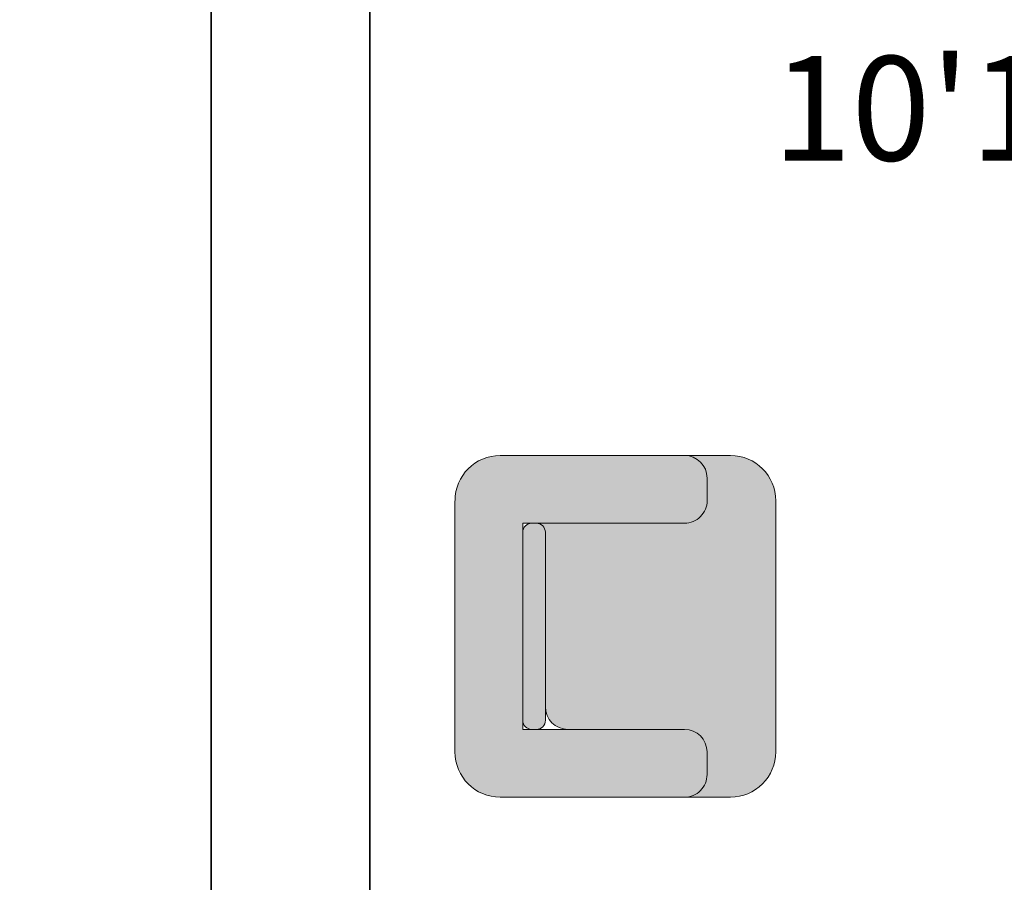
# Model space of a CAD drawing. Units: millimetres. Extents: x 27017497 to 27018854, y 7058029 to 7059154.
# Tile 33 of 91: x 27017621 to 27017677, y 7058337 to 7058386. Entities that reach past the tile are written whole.
import ezdxf

# ---------------------------------------------------------------- set-up
doc = ezdxf.new("R2010")
doc.units = ezdxf.units.MM
for name, color, linetype, lineweight in [('A-ANNO-DIMS', 2, 'Continuous', 18), ('A-FURN', 8, 'Continuous', 18), ('A-WALL', 7, 'Continuous', 35)]:
    doc.layers.add(name, color=color, linetype=linetype, lineweight=lineweight)
doc.layers.add('A-FURN-PATT', color=177, linetype='Continuous', lineweight=13, true_color=0x293189)
doc.styles.get("Standard").update_dxf_attribs({"font": 'arial.ttf'})
doc.dimstyles.get("Standard").update_dxf_attribs({"dimtxt": 0.18, "dimasz": 0.18, "dimexe": 0.18, "dimexo": 0.0625, "dimgap": 0.09, "dimtad": 0, "dimtih": 1, "dimtoh": 1, "dimdec": 4, "dimzin": 0, "dimdsep": 46, "dimtxsty": 'Standard', "dimcen": 0.09, "dimadec": 0, "dimazin": 0, "dimtfac": 1, "dimtdec": 4, "dimtofl": 0, "dimtmove": 0, "dimatfit": 3, "dimfxl": 1, "dimtolj": 1, "dimtzin": 0, "dimarcsym": 0})

# ---------------------------------------------------------------- blocks, each defined once
blk = doc.blocks.new('CHAIR-OCCASIONAL')
for p, q in [((19.599, 18.742), (7.02, 22.21)), ((3.873, 20.423), (0.092, 6.706)), ((4.132, 6.919), (7.234, 18.169)), ((5.25, 10.974), (7.234, 18.169)), ((16.064, 15.735), (7.234, 18.169)), ((7.234, 18.169), (16.064, 15.735)), ((7.234, 18.169), (16.064, 15.735)), ((7.727, 18.033), (7.974, 17.965)), ((7.727, 18.033), (7.974, 17.965)), ((17.638, 16.628), (17.978, 17.862)), ((17.638, 16.628), (17.978, 17.862)), ((5.25, 10.974), (7.098, 17.676)), ((8.331, 17.336), (5.625, 7.52)), ((17.605, 1.878), (21.386, 15.595)), ((5.625, 7.52), (5.502, 7.072)), ((12.963, 4.485), (4.132, 6.919)), ((4.872, 6.715), (4.626, 6.783)), ((1.879, 3.558), (14.458, 0.091)), ((13.856, 2.911), (13.516, 1.678))]:
    blk.add_line(p, q)
for centre, radius, start, end in [((6.34, 19.743), 2.559, 74.5879, 164.5879), ((16.744, 18.202), 1.28, 344.5879, 74.5879), ((16.744, 18.202), 1.28, 344.5879, 74.5879), ((18.919, 16.275), 2.559, 344.5879, 74.5879), ((7.591, 17.54), 0.512, 74.5879, 164.5879), ((7.838, 17.472), 0.512, 344.5879, 74.5879), ((9.361, 16.256), 1.28, 74.5879, 164.5879), ((16.404, 16.968), 1.28, 254.5879, 344.5879), ((16.404, 16.968), 1.28, 254.5879, 344.5879), ((4.762, 7.276), 0.512, 164.5879, 254.5879), ((2.559, 6.025), 2.559, 164.5879, 254.5879), ((5.008, 7.208), 0.512, 254.5879, 344.5879), ((12.623, 3.251), 1.28, 344.5879, 74.5879), ((12.283, 2.018), 1.28, 254.5879, 344.5879), ((15.138, 2.558), 2.559, 254.5879, 344.5879)]:
    blk.add_arc(centre, radius, start, end)
blk = doc.blocks.new('*D48')
at = {"layer": 'A-ANNO-DIMS', "color": 0, "lineweight": -2, "transparency": 16777216}
for p, q in [((27018463.498, 7058622.912), (27017497.536, 7058622.912)), ((27017497.716, 7058622.732), (27017497.716, 7058357.753)), ((27017497.716, 7058092.41), (27017497.716, 7058357.389)), ((27018555.129, 7058092.23), (27017497.536, 7058092.23))]:
    blk.add_line(p, q, dxfattribs=at)
at = {"layer": 'A-ANNO-DIMS', "color": 0, "transparency": 16777216}
for points in [[(27017497.686, 7058622.732), (27017497.746, 7058622.732), (27017497.716, 7058622.912)], [(27017497.686, 7058092.41), (27017497.746, 7058092.41), (27017497.716, 7058092.23)]]:
    blk.add_solid(points, dxfattribs=at)
at = {"layer": 'Defpoints', "color": 0, "transparency": 16777216}
for p in [(27018463.561, 7058622.912), (27017497.716, 7058092.23), (27018555.192, 7058092.23)]:
    blk.add_point(p, dxfattribs=at)
at = {"layer": 'A-ANNO-DIMS', "color": 0, "transparency": 16777216, "insert": (27017497.716, 7058357.571), "char_height": 0.18, "attachment_point": 5}
blk.add_mtext('\\A1;530.7', dxfattribs=at)

msp = doc.modelspace()

# ---------------------------------------------------------------- hatches: boundary and pattern name
at = {"layer": 'A-FURN-PATT'}
h = msp.add_hatch(color=256, dxfattribs=at)
h.dxf.hatch_style = 1
h.paths.add_polyline_path([(27017716.96, 7058359.767), (27017683.615, 7058359.767), (27017683.615, 7058343.095), (27017716.96, 7058343.095)])
h.paths.add_polyline_path([(27017716.127, 7058358.933), (27017716.127, 7058343.928), (27017684.449, 7058343.928), (27017684.449, 7058358.933)], flags=16)
h.paths.add_polyline_path([(27017660.259, 7058359.819, 0.414214), (27017658.98, 7058361.098), (27017648.54, 7058361.098, 0.414214), (27017645.981, 7058358.539), (27017645.981, 7058344.31, 0.414214), (27017648.54, 7058341.751), (27017658.98, 7058341.751, 0.414214), (27017660.259, 7058343.031), (27017660.259, 7058344.31, 0.414214), (27017658.98, 7058345.59), (27017649.82, 7058345.59), (27017649.82, 7058353.053), (27017649.82, 7058357.26), (27017658.98, 7058357.26, 0.414214), (27017660.259, 7058358.539)])
h.paths.add_polyline_path([(27017664.147, 7058358.539, 0.414214), (27017661.588, 7058361.098), (27017658.98, 7058361.098, -0.414214), (27017660.259, 7058359.819), (27017660.259, 7058358.539, -0.414214), (27017658.98, 7058357.26), (27017650.587, 7058357.26, -0.414214), (27017651.099, 7058356.748), (27017651.099, 7058356.283), (27017651.099, 7058346.869, 0.414214), (27017652.379, 7058345.59), (27017658.98, 7058345.59, -0.414214), (27017660.259, 7058344.31), (27017660.259, 7058343.031, -0.414214), (27017658.98, 7058341.751), (27017661.588, 7058341.751, 0.414214), (27017664.147, 7058344.31)])
h.paths.add_polyline_path([(27017651.099, 7058356.283), (27017651.099, 7058356.748, 0.414214), (27017650.587, 7058357.26), (27017650.331, 7058357.26, 0.414214), (27017649.82, 7058356.748), (27017649.82, 7058346.101, 0.414214), (27017650.331, 7058345.59), (27017650.587, 7058345.59, 0.414214), (27017651.099, 7058346.101)], flags=17)

# ---------------------------------------------------------------- linework, layer by layer
at = {"layer": 'A-WALL'}
for p, q in [((27017632.166, 7058432.412), (27017632.166, 7058298.912)), ((27017641.166, 7058432.412), (27017641.166, 7058298.912))]:
    msp.add_line(p, q, dxfattribs=at)

# ---------------------------------------------------------------- block references
at = {"layer": 'A-FURN', "extrusion": (0, 0, -1), "zscale": -1, "rotation": 195.4121391531662}
msp.add_blockref('CHAIR-OCCASIONAL', (-27017647.675, 7058365.028), dxfattribs=at)

# ---------------------------------------------------------------- texts
at = {"layer": 'A-ANNO-DIMS'}
msp.add_text('10\'1"X11\'6"', height=5.91176, dxfattribs=at).set_placement((27017663.959, 7058377.8))

# ---------------------------------------------------------------- dimensions: what is measured, and where the dimension line sits
dim = msp.add_linear_dim(base=(27017497.716, 7058092.23), p1=(27018463.561, 7058622.912), p2=(27018555.192, 7058092.23), angle=90, dimstyle='Standard', override={"dimdec": 1, "dimlfac": 1, "dimrnd": 0, "dimzin": 0, "dimdsep": 46, "dimlunit": 2}, dxfattribs=at)
dim.commit()
dim.dimension.update_dxf_attribs({"geometry": '*D48', "text_midpoint": (27017497.716, 7058357.571)})

doc.saveas('drawing.dxf')
